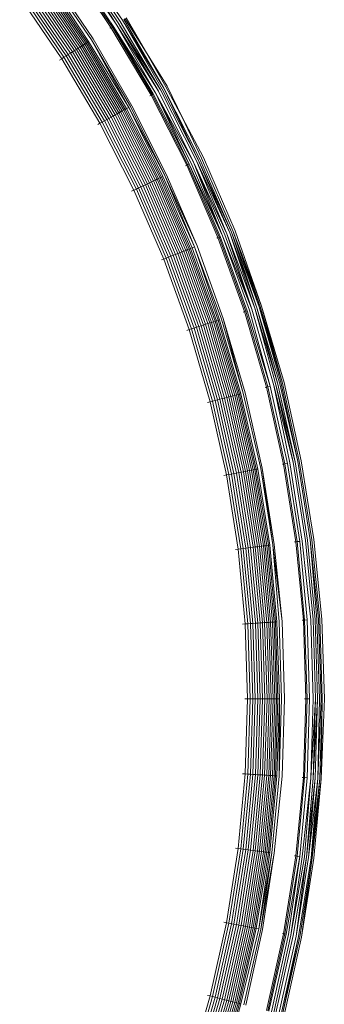
# Model space of a CAD drawing. Units: inches. Extents: x 64 to 1167, y 117 to 939.
# Tile 53 of 56: x 1131.1131 to 1131.3839, y 500.6716 to 501.5456. Entities that reach past the tile are written whole.
import ezdxf

# ---------------------------------------------------------------- set-up
doc = ezdxf.new("R2010")
doc.units = ezdxf.units.IN
doc.header["$MEASUREMENT"] = 0
doc.layers.add('A-FLOR-FIXT', color=8, linetype='Continuous', lineweight=18)

msp = doc.modelspace()

# ---------------------------------------------------------------- linework, layer by layer
at = {"layer": 'A-FLOR-FIXT'}
for p, q in [((1131.20239, 501.54385), (1131.1635, 501.60266)), ((1131.20452, 501.5452), (1131.16482, 501.60362)), ((1131.1943, 501.53871), (1131.15502, 501.5965)), ((1131.19527, 501.53932), (1131.15595, 501.59718)), ((1131.19623, 501.53993), (1131.15687, 501.59785)), ((1131.19902, 501.54171), (1131.15955, 501.59979)), ((1131.19902, 501.54171), (1131.16123, 501.60101)), ((1131.20077, 501.54282), (1131.16123, 501.60101)), ((1131.17837, 501.5286), (1131.13976, 501.58542)), ((1131.1652, 501.52024), (1131.12714, 501.57624)), ((1131.16678, 501.52125), (1131.12865, 501.57735)), ((1131.16829, 501.5222), (1131.1301, 501.57839)), ((1131.16971, 501.52311), (1131.13146, 501.57939)), ((1131.17104, 501.52395), (1131.13274, 501.58031)), ((1131.17228, 501.52474), (1131.13393, 501.58117)), ((1131.17342, 501.52546), (1131.13501, 501.58197)), ((1131.17445, 501.52611), (1131.13688, 501.58332)), ((1131.17686, 501.52764), (1131.13831, 501.58436)), ((1131.15253, 501.5122), (1131.115, 501.56742)), ((1131.15445, 501.51342), (1131.11684, 501.56876)), ((1131.15635, 501.51463), (1131.11866, 501.57009)), ((1131.15822, 501.51581), (1131.12045, 501.57139)), ((1131.16004, 501.51697), (1131.1222, 501.57266)), ((1131.16182, 501.5181), (1131.1239, 501.57389)), ((1131.16354, 501.51919), (1131.12555, 501.57509)), ((1131.15059, 501.51097), (1131.11314, 501.56607)), ((1131.23383, 501.48074), (1131.19902, 501.54171)), ((1131.23659, 501.48226), (1131.19902, 501.54171)), ((1131.23827, 501.48318), (1131.20077, 501.54282)), ((1131.23659, 501.48226), (1131.20077, 501.54282)), ((1131.23827, 501.48318), (1131.20239, 501.54385)), ((1131.23979, 501.48402), (1131.20452, 501.5452)), ((1131.24112, 501.48475), (1131.20452, 501.5452)), ((1131.24112, 501.48475), (1131.20571, 501.54595)), ((1131.22483, 501.51757), (1131.20669, 501.54657)), ((1131.22483, 501.51757), (1131.20771, 501.54722)), ((1131.19332, 501.53809), (1131.1943, 501.53871)), ((1131.1943, 501.53871), (1131.19527, 501.53932)), ((1131.22987, 501.47856), (1131.1943, 501.53871)), ((1131.19527, 501.53932), (1131.19623, 501.53993)), ((1131.23087, 501.47912), (1131.19527, 501.53932)), ((1131.23187, 501.47967), (1131.19623, 501.53993)), ((1131.23383, 501.48074), (1131.19623, 501.53993)), ((1131.16971, 501.52311), (1131.17104, 501.52395)), ((1131.17104, 501.52395), (1131.17228, 501.52474)), ((1131.20573, 501.46529), (1131.17104, 501.52395)), ((1131.17228, 501.52474), (1131.17342, 501.52546)), ((1131.20702, 501.466), (1131.17228, 501.52474)), ((1131.17342, 501.52546), (1131.17445, 501.52611)), ((1131.2082, 501.46665), (1131.17342, 501.52546)), ((1131.21022, 501.46776), (1131.17445, 501.52611)), ((1131.21177, 501.46861), (1131.17686, 501.52764)), ((1131.21022, 501.46776), (1131.17686, 501.52764)), ((1131.21281, 501.46919), (1131.17837, 501.5286)), ((1131.15635, 501.51463), (1131.15822, 501.51581)), ((1131.15822, 501.51581), (1131.16004, 501.51697)), ((1131.19242, 501.45798), (1131.15822, 501.51581)), ((1131.16004, 501.51697), (1131.16182, 501.5181)), ((1131.19432, 501.45902), (1131.16004, 501.51697)), ((1131.16182, 501.5181), (1131.16354, 501.51919)), ((1131.19616, 501.46003), (1131.16182, 501.5181)), ((1131.16354, 501.51919), (1131.1652, 501.52024)), ((1131.19794, 501.46101), (1131.16354, 501.51919)), ((1131.1652, 501.52024), (1131.16678, 501.52125)), ((1131.19966, 501.46196), (1131.1652, 501.52024)), ((1131.16678, 501.52125), (1131.16829, 501.5222)), ((1131.20131, 501.46286), (1131.16678, 501.52125)), ((1131.16829, 501.5222), (1131.16971, 501.52311)), ((1131.20287, 501.46372), (1131.16829, 501.5222)), ((1131.20435, 501.46453), (1131.16971, 501.52311)), ((1131.24314, 501.48586), (1131.22483, 501.51757)), ((1131.24429, 501.48649), (1131.22483, 501.51757)), ((1131.14864, 501.50973), (1131.15059, 501.51097)), ((1131.15059, 501.51097), (1131.15253, 501.5122)), ((1131.1845, 501.45362), (1131.15059, 501.51097)), ((1131.15445, 501.51342), (1131.15253, 501.5122)), ((1131.18652, 501.45473), (1131.15253, 501.5122)), ((1131.15445, 501.51342), (1131.15635, 501.51463)), ((1131.18851, 501.45583), (1131.15445, 501.51342)), ((1131.19049, 501.45691), (1131.15635, 501.51463)), ((1131.26761, 501.41913), (1131.23383, 501.48074)), ((1131.26568, 501.41823), (1131.23383, 501.48074)), ((1131.26366, 501.41728), (1131.23383, 501.48074)), ((1131.26761, 501.41913), (1131.23659, 501.48226)), ((1131.27027, 501.42038), (1131.23827, 501.48318)), ((1131.27184, 501.42112), (1131.23979, 501.48402)), ((1131.27321, 501.42177), (1131.24112, 501.48475)), ((1131.27184, 501.42112), (1131.24112, 501.48475)), ((1131.25772, 501.45841), (1131.24314, 501.48586)), ((1131.25772, 501.45841), (1131.24429, 501.48649)), ((1131.22987, 501.47856), (1131.22886, 501.47801)), ((1131.23087, 501.47912), (1131.22987, 501.47856)), ((1131.26159, 501.4163), (1131.22987, 501.47856)), ((1131.23187, 501.47967), (1131.23087, 501.47912)), ((1131.26263, 501.41679), (1131.23087, 501.47912)), ((1131.26366, 501.41728), (1131.23187, 501.47967)), ((1131.20131, 501.46286), (1131.19966, 501.46196)), ((1131.20287, 501.46372), (1131.20131, 501.46286)), ((1131.2321, 501.40243), (1131.20131, 501.46286)), ((1131.20435, 501.46453), (1131.20287, 501.46372)), ((1131.23372, 501.40319), (1131.20287, 501.46372)), ((1131.20573, 501.46529), (1131.20435, 501.46453)), ((1131.23524, 501.4039), (1131.20435, 501.46453)), ((1131.20702, 501.466), (1131.20573, 501.46529)), ((1131.23667, 501.40458), (1131.20573, 501.46529)), ((1131.2082, 501.46665), (1131.20702, 501.466)), ((1131.238, 501.4052), (1131.20702, 501.466)), ((1131.21022, 501.46776), (1131.2082, 501.46665)), ((1131.23921, 501.40577), (1131.2082, 501.46665)), ((1131.24216, 501.40716), (1131.21022, 501.46776)), ((1131.24032, 501.40629), (1131.21022, 501.46776)), ((1131.24216, 501.40716), (1131.21177, 501.46861)), ((1131.24351, 501.40779), (1131.21281, 501.46919)), ((1131.18652, 501.45473), (1131.1845, 501.45362)), ((1131.18851, 501.45583), (1131.18652, 501.45473)), ((1131.21683, 501.39524), (1131.18652, 501.45473)), ((1131.19049, 501.45691), (1131.18851, 501.45583)), ((1131.21889, 501.39621), (1131.18851, 501.45583)), ((1131.19242, 501.45798), (1131.19049, 501.45691)), ((1131.22093, 501.39717), (1131.19049, 501.45691)), ((1131.19432, 501.45902), (1131.19242, 501.45798)), ((1131.22293, 501.39811), (1131.19242, 501.45798)), ((1131.19616, 501.46003), (1131.19432, 501.45902)), ((1131.22488, 501.39903), (1131.19432, 501.45902)), ((1131.19794, 501.46101), (1131.19616, 501.46003)), ((1131.22679, 501.39992), (1131.19616, 501.46003)), ((1131.19966, 501.46196), (1131.19794, 501.46101)), ((1131.22863, 501.40079), (1131.19794, 501.46101)), ((1131.2304, 501.40163), (1131.19966, 501.46196)), ((1131.27487, 501.42255), (1131.25772, 501.45841)), ((1131.27638, 501.42326), (1131.25772, 501.45841)), ((1131.1845, 501.45362), (1131.18248, 501.45251)), ((1131.21475, 501.39426), (1131.1845, 501.45362)), ((1131.29738, 501.35536), (1131.26761, 501.41913)), ((1131.29354, 501.35384), (1131.26761, 501.41913)), ((1131.29553, 501.35462), (1131.26761, 501.41913)), ((1131.29738, 501.35536), (1131.27027, 501.42038)), ((1131.29987, 501.35634), (1131.27027, 501.42038)), ((1131.29987, 501.35634), (1131.27184, 501.42112)), ((1131.30129, 501.3569), (1131.27184, 501.42112)), ((1131.30129, 501.3569), (1131.27321, 501.42177)), ((1131.30298, 501.35757), (1131.27487, 501.42255)), ((1131.30468, 501.35824), (1131.27638, 501.42326)), ((1131.26159, 501.4163), (1131.26055, 501.41581)), ((1131.26263, 501.41679), (1131.26159, 501.4163)), ((1131.28934, 501.35217), (1131.26159, 501.4163)), ((1131.26366, 501.41728), (1131.26263, 501.41679)), ((1131.29041, 501.3526), (1131.26263, 501.41679)), ((1131.29354, 501.35384), (1131.26366, 501.41728)), ((1131.29147, 501.35302), (1131.26366, 501.41728)), ((1131.29354, 501.35384), (1131.26568, 501.41823)), ((1131.2304, 501.40163), (1131.22863, 501.40079)), ((1131.2321, 501.40243), (1131.2304, 501.40163)), ((1131.25729, 501.33948), (1131.2304, 501.40163)), ((1131.23372, 501.40319), (1131.2321, 501.40243)), ((1131.25904, 501.34018), (1131.2321, 501.40243)), ((1131.23524, 501.4039), (1131.23372, 501.40319)), ((1131.2607, 501.34083), (1131.23372, 501.40319)), ((1131.23667, 501.40458), (1131.23524, 501.4039)), ((1131.26227, 501.34145), (1131.23524, 501.4039)), ((1131.238, 501.4052), (1131.23667, 501.40458)), ((1131.26374, 501.34203), (1131.23667, 501.40458)), ((1131.23921, 501.40577), (1131.238, 501.4052)), ((1131.2651, 501.34257), (1131.238, 501.4052)), ((1131.24032, 501.40629), (1131.23921, 501.40577)), ((1131.26635, 501.34307), (1131.23921, 501.40577)), ((1131.26849, 501.34392), (1131.24032, 501.40629)), ((1131.26849, 501.34392), (1131.24216, 501.40716)), ((1131.27076, 501.34482), (1131.24216, 501.40716)), ((1131.27076, 501.34482), (1131.24351, 501.40779)), ((1131.21475, 501.39426), (1131.21266, 501.39328)), ((1131.21683, 501.39524), (1131.21475, 501.39426)), ((1131.24121, 501.33312), (1131.21475, 501.39426)), ((1131.21889, 501.39621), (1131.21683, 501.39524)), ((1131.24335, 501.33396), (1131.21683, 501.39524)), ((1131.22093, 501.39717), (1131.21889, 501.39621)), ((1131.24547, 501.3348), (1131.21889, 501.39621)), ((1131.22293, 501.39811), (1131.22093, 501.39717)), ((1131.24756, 501.33563), (1131.22093, 501.39717)), ((1131.22488, 501.39903), (1131.22293, 501.39811)), ((1131.24961, 501.33644), (1131.22293, 501.39811)), ((1131.22679, 501.39992), (1131.22488, 501.39903)), ((1131.25162, 501.33724), (1131.22488, 501.39903)), ((1131.22863, 501.40079), (1131.22679, 501.39992)), ((1131.25358, 501.33801), (1131.22679, 501.39992)), ((1131.25547, 501.33876), (1131.22863, 501.40079)), ((1131.32587, 501.2906), (1131.30298, 501.35757)), ((1131.32697, 501.29096), (1131.30298, 501.35757)), ((1131.32812, 501.29134), (1131.30298, 501.35757)), ((1131.32812, 501.29134), (1131.30468, 501.35824)), ((1131.28827, 501.35175), (1131.28934, 501.35217)), ((1131.28934, 501.35217), (1131.29041, 501.3526)), ((1131.31301, 501.28643), (1131.28934, 501.35217)), ((1131.29041, 501.3526), (1131.29147, 501.35302)), ((1131.3141, 501.28678), (1131.29041, 501.3526)), ((1131.31519, 501.28713), (1131.29147, 501.35302)), ((1131.31731, 501.28782), (1131.29354, 501.35384)), ((1131.31934, 501.28848), (1131.29354, 501.35384)), ((1131.31934, 501.28848), (1131.29553, 501.35462)), ((1131.31934, 501.28848), (1131.29738, 501.35536)), ((1131.32213, 501.28939), (1131.29738, 501.35536)), ((1131.32378, 501.28993), (1131.29987, 501.35634)), ((1131.32213, 501.28939), (1131.29987, 501.35634)), ((1131.32587, 501.2906), (1131.30129, 501.3569)), ((1131.32378, 501.28993), (1131.30129, 501.3569)), ((1131.25729, 501.33948), (1131.25904, 501.34018)), ((1131.25904, 501.34018), (1131.2607, 501.34083)), ((1131.28202, 501.27636), (1131.25904, 501.34018)), ((1131.2607, 501.34083), (1131.26227, 501.34145)), ((1131.28371, 501.27691), (1131.2607, 501.34083)), ((1131.26227, 501.34145), (1131.26374, 501.34203)), ((1131.28532, 501.27743), (1131.26227, 501.34145)), ((1131.26374, 501.34203), (1131.2651, 501.34257)), ((1131.28682, 501.27792), (1131.26374, 501.34203)), ((1131.2651, 501.34257), (1131.26635, 501.34307)), ((1131.28821, 501.27837), (1131.2651, 501.34257)), ((1131.26635, 501.34307), (1131.26849, 501.34392)), ((1131.28949, 501.27879), (1131.26635, 501.34307)), ((1131.29065, 501.27916), (1131.26849, 501.34392)), ((1131.29259, 501.27979), (1131.26849, 501.34392)), ((1131.294, 501.28025), (1131.27076, 501.34482)), ((1131.24121, 501.33312), (1131.23906, 501.33227)), ((1131.24335, 501.33396), (1131.24121, 501.33312)), ((1131.26378, 501.27043), (1131.24121, 501.33312)), ((1131.24547, 501.3348), (1131.24335, 501.33396)), ((1131.26596, 501.27114), (1131.24335, 501.33396)), ((1131.24756, 501.33563), (1131.24547, 501.3348)), ((1131.26813, 501.27185), (1131.24547, 501.3348)), ((1131.24961, 501.33644), (1131.24756, 501.33563)), ((1131.27027, 501.27254), (1131.24756, 501.33563)), ((1131.24961, 501.33644), (1131.25162, 501.33724)), ((1131.27237, 501.27322), (1131.24961, 501.33644)), ((1131.25162, 501.33724), (1131.25358, 501.33801)), ((1131.27443, 501.27389), (1131.25162, 501.33724)), ((1131.25358, 501.33801), (1131.25547, 501.33876)), ((1131.27643, 501.27454), (1131.25358, 501.33801)), ((1131.25547, 501.33876), (1131.25729, 501.33948)), ((1131.27837, 501.27517), (1131.25547, 501.33876)), ((1131.28023, 501.27578), (1131.25729, 501.33948)), ((1131.33581, 501.22017), (1131.31731, 501.28782)), ((1131.33895, 501.22098), (1131.31934, 501.28848)), ((1131.34266, 501.22193), (1131.32213, 501.28939)), ((1131.34088, 501.22148), (1131.32213, 501.28939)), ((1131.34266, 501.22193), (1131.32378, 501.28993)), ((1131.34424, 501.22234), (1131.32378, 501.28993)), ((1131.3456, 501.22269), (1131.32587, 501.2906)), ((1131.34672, 501.22297), (1131.32587, 501.2906)), ((1131.34672, 501.22297), (1131.32697, 501.29096)), ((1131.34833, 501.22339), (1131.32812, 501.29134)), ((1131.34672, 501.22297), (1131.32812, 501.29134)), ((1131.29065, 501.27916), (1131.28949, 501.27879)), ((1131.30973, 501.21348), (1131.29065, 501.27916)), ((1131.31171, 501.21399), (1131.29259, 501.27979)), ((1131.31366, 501.21449), (1131.294, 501.28025)), ((1131.31171, 501.21399), (1131.294, 501.28025)), ((1131.31301, 501.28643), (1131.31191, 501.28607)), ((1131.31301, 501.28643), (1131.3141, 501.28678)), ((1131.33251, 501.21933), (1131.31301, 501.28643)), ((1131.3141, 501.28678), (1131.31519, 501.28713)), ((1131.33362, 501.21961), (1131.3141, 501.28678)), ((1131.33581, 501.22017), (1131.31519, 501.28713)), ((1131.26158, 501.26972), (1131.26378, 501.27043)), ((1131.26378, 501.27043), (1131.26596, 501.27114)), ((1131.28237, 501.20645), (1131.26378, 501.27043)), ((1131.26596, 501.27114), (1131.26813, 501.27185)), ((1131.28459, 501.20702), (1131.26596, 501.27114)), ((1131.26813, 501.27185), (1131.27027, 501.27254)), ((1131.2868, 501.20759), (1131.26813, 501.27185)), ((1131.27027, 501.27254), (1131.27237, 501.27322)), ((1131.28898, 501.20815), (1131.27027, 501.27254)), ((1131.27237, 501.27322), (1131.27443, 501.27389)), ((1131.29112, 501.2087), (1131.27237, 501.27322)), ((1131.27643, 501.27454), (1131.27443, 501.27389)), ((1131.29321, 501.20924), (1131.27443, 501.27389)), ((1131.27837, 501.27517), (1131.27643, 501.27454)), ((1131.29525, 501.20976), (1131.27643, 501.27454)), ((1131.28023, 501.27578), (1131.27837, 501.27517)), ((1131.29722, 501.21027), (1131.27837, 501.27517)), ((1131.28202, 501.27636), (1131.28023, 501.27578)), ((1131.29912, 501.21075), (1131.28023, 501.27578)), ((1131.28371, 501.27691), (1131.28202, 501.27636)), ((1131.30094, 501.21122), (1131.28202, 501.27636)), ((1131.28532, 501.27743), (1131.28371, 501.27691)), ((1131.30267, 501.21166), (1131.28371, 501.27691)), ((1131.28682, 501.27792), (1131.28532, 501.27743)), ((1131.3043, 501.21208), (1131.28532, 501.27743)), ((1131.28821, 501.27837), (1131.28682, 501.27792)), ((1131.30583, 501.21248), (1131.28682, 501.27792)), ((1131.28949, 501.27879), (1131.28821, 501.27837)), ((1131.30725, 501.21284), (1131.28821, 501.27837)), ((1131.30855, 501.21318), (1131.28949, 501.27879)), ((1131.33251, 501.21933), (1131.33139, 501.21904)), ((1131.33362, 501.21961), (1131.33251, 501.21933)), ((1131.34775, 501.15113), (1131.33251, 501.21933)), ((1131.33581, 501.22017), (1131.33362, 501.21961)), ((1131.34888, 501.15135), (1131.33362, 501.21961)), ((1131.3511, 501.15177), (1131.33581, 501.22017)), ((1131.35625, 501.15275), (1131.33895, 501.22098)), ((1131.35325, 501.15218), (1131.33895, 501.22098)), ((1131.35625, 501.15275), (1131.34088, 501.22148)), ((1131.35804, 501.1531), (1131.34088, 501.22148)), ((1131.35804, 501.1531), (1131.34266, 501.22193)), ((1131.36037, 501.15354), (1131.34424, 501.22234)), ((1131.36037, 501.15354), (1131.3456, 501.22269)), ((1131.36163, 501.15378), (1131.34672, 501.22297)), ((1131.36336, 501.15411), (1131.34833, 501.22339)), ((1131.29112, 501.2087), (1131.29321, 501.20924)), ((1131.29321, 501.20924), (1131.29525, 501.20976)), ((1131.3079, 501.14353), (1131.29321, 501.20924)), ((1131.29525, 501.20976), (1131.29722, 501.21027)), ((1131.30997, 501.14392), (1131.29525, 501.20976)), ((1131.29722, 501.21027), (1131.29912, 501.21075)), ((1131.31197, 501.14431), (1131.29722, 501.21027)), ((1131.29912, 501.21075), (1131.30094, 501.21122)), ((1131.31389, 501.14467), (1131.29912, 501.21075)), ((1131.30094, 501.21122), (1131.30267, 501.21166)), ((1131.31574, 501.14503), (1131.30094, 501.21122)), ((1131.30267, 501.21166), (1131.3043, 501.21208)), ((1131.31749, 501.14536), (1131.30267, 501.21166)), ((1131.3043, 501.21208), (1131.30583, 501.21248)), ((1131.31915, 501.14568), (1131.3043, 501.21208)), ((1131.30583, 501.21248), (1131.30725, 501.21284)), ((1131.3207, 501.14597), (1131.30583, 501.21248)), ((1131.30725, 501.21284), (1131.30855, 501.21318)), ((1131.32214, 501.14625), (1131.30725, 501.21284)), ((1131.30855, 501.21318), (1131.30973, 501.21348)), ((1131.32346, 501.1465), (1131.30855, 501.21318)), ((1131.32466, 501.14673), (1131.30973, 501.21348)), ((1131.32746, 501.14726), (1131.31171, 501.21399)), ((1131.32863, 501.14749), (1131.31366, 501.21449)), ((1131.28013, 501.20588), (1131.28237, 501.20645)), ((1131.28237, 501.20645), (1131.28459, 501.20702)), ((1131.2969, 501.14143), (1131.28237, 501.20645)), ((1131.28459, 501.20702), (1131.2868, 501.20759)), ((1131.29916, 501.14186), (1131.28459, 501.20702)), ((1131.2868, 501.20759), (1131.28898, 501.20815)), ((1131.3014, 501.14229), (1131.2868, 501.20759)), ((1131.28898, 501.20815), (1131.29112, 501.2087)), ((1131.30361, 501.14271), (1131.28898, 501.20815)), ((1131.30578, 501.14313), (1131.29112, 501.2087)), ((1131.34662, 501.15092), (1131.34775, 501.15113)), ((1131.34775, 501.15113), (1131.34888, 501.15135)), ((1131.35868, 501.08212), (1131.34775, 501.15113)), ((1131.34888, 501.15135), (1131.3511, 501.15177)), ((1131.35982, 501.08226), (1131.34888, 501.15135)), ((1131.36207, 501.08254), (1131.3511, 501.15177)), ((1131.36424, 501.08282), (1131.35325, 501.15218)), ((1131.36726, 501.0832), (1131.35625, 501.15275)), ((1131.36908, 501.08343), (1131.35804, 501.1531)), ((1131.37143, 501.08373), (1131.36037, 501.15354)), ((1131.3727, 501.08389), (1131.36163, 501.15378)), ((1131.37445, 501.08411), (1131.36336, 501.15411)), ((1131.2969, 501.14143), (1131.29463, 501.141)), ((1131.29916, 501.14186), (1131.2969, 501.14143)), ((1131.30732, 501.07563), (1131.2969, 501.14143)), ((1131.3014, 501.14229), (1131.29916, 501.14186)), ((1131.3096, 501.07592), (1131.29916, 501.14186)), ((1131.30361, 501.14271), (1131.3014, 501.14229)), ((1131.31186, 501.0762), (1131.3014, 501.14229)), ((1131.30578, 501.14313), (1131.30361, 501.14271)), ((1131.31409, 501.07648), (1131.30361, 501.14271)), ((1131.3079, 501.14353), (1131.30578, 501.14313)), ((1131.31629, 501.07676), (1131.30578, 501.14313)), ((1131.30997, 501.14392), (1131.3079, 501.14353)), ((1131.31843, 501.07703), (1131.3079, 501.14353)), ((1131.31197, 501.14431), (1131.30997, 501.14392)), ((1131.32052, 501.07729), (1131.30997, 501.14392)), ((1131.31389, 501.14467), (1131.31197, 501.14431)), ((1131.32254, 501.07755), (1131.31197, 501.14431)), ((1131.31574, 501.14503), (1131.31389, 501.14467)), ((1131.32448, 501.0778), (1131.31389, 501.14467)), ((1131.31749, 501.14536), (1131.31574, 501.14503)), ((1131.32635, 501.07803), (1131.31574, 501.14503)), ((1131.31915, 501.14568), (1131.31749, 501.14536)), ((1131.32812, 501.07825), (1131.31749, 501.14536)), ((1131.3207, 501.14597), (1131.31915, 501.14568)), ((1131.32979, 501.07847), (1131.31915, 501.14568)), ((1131.32214, 501.14625), (1131.3207, 501.14597)), ((1131.33136, 501.07866), (1131.3207, 501.14597)), ((1131.32346, 501.1465), (1131.32214, 501.14625)), ((1131.33281, 501.07885), (1131.32214, 501.14625)), ((1131.32466, 501.14673), (1131.32346, 501.1465)), ((1131.33415, 501.07902), (1131.32346, 501.1465)), ((1131.33536, 501.07917), (1131.32466, 501.14673)), ((1131.33819, 501.07953), (1131.32746, 501.14726)), ((1131.33937, 501.07968), (1131.32863, 501.14749)), ((1131.33819, 501.07953), (1131.32863, 501.14749)), ((1131.32448, 501.0778), (1131.32635, 501.07803)), ((1131.32635, 501.07803), (1131.32812, 501.07825)), ((1131.33273, 501.0105), (1131.32635, 501.07803)), ((1131.32812, 501.07825), (1131.32979, 501.07847)), ((1131.33451, 501.01062), (1131.32812, 501.07825)), ((1131.32979, 501.07847), (1131.33136, 501.07866)), ((1131.33619, 501.01072), (1131.32979, 501.07847)), ((1131.33136, 501.07866), (1131.33281, 501.07885)), ((1131.33777, 501.01082), (1131.33136, 501.07866)), ((1131.33281, 501.07885), (1131.33415, 501.07902)), ((1131.33923, 501.01091), (1131.33281, 501.07885)), ((1131.33415, 501.07902), (1131.33536, 501.07917)), ((1131.34058, 501.011), (1131.33415, 501.07902)), ((1131.34179, 501.01107), (1131.33536, 501.07917)), ((1131.34383, 501.0112), (1131.33819, 501.07953)), ((1131.34644, 501.01137), (1131.33819, 501.07953)), ((1131.34644, 501.01137), (1131.33937, 501.07968)), ((1131.35868, 501.08212), (1131.35754, 501.08197)), ((1131.35982, 501.08226), (1131.35868, 501.08212)), ((1131.36526, 501.01255), (1131.35868, 501.08212)), ((1131.36207, 501.08254), (1131.35982, 501.08226)), ((1131.3664, 501.01262), (1131.35982, 501.08226)), ((1131.36866, 501.01276), (1131.36207, 501.08254)), ((1131.37189, 501.01297), (1131.36424, 501.08282)), ((1131.37389, 501.01309), (1131.36726, 501.0832)), ((1131.37572, 501.01321), (1131.36908, 501.08343)), ((1131.37735, 501.01331), (1131.37143, 501.08373)), ((1131.37875, 501.0134), (1131.37143, 501.08373)), ((1131.3799, 501.01347), (1131.3727, 501.08389)), ((1131.38168, 501.01358), (1131.37445, 501.08411)), ((1131.30732, 501.07563), (1131.30503, 501.07534)), ((1131.3096, 501.07592), (1131.30732, 501.07563)), ((1131.31359, 501.0093), (1131.30732, 501.07563)), ((1131.31186, 501.0762), (1131.3096, 501.07592)), ((1131.31589, 501.00944), (1131.3096, 501.07592)), ((1131.31186, 501.0762), (1131.31409, 501.07648)), ((1131.31816, 501.00959), (1131.31186, 501.0762)), ((1131.31409, 501.07648), (1131.31629, 501.07676)), ((1131.3204, 501.00973), (1131.31409, 501.07648)), ((1131.31629, 501.07676), (1131.31843, 501.07703)), ((1131.32261, 501.00987), (1131.31629, 501.07676)), ((1131.31843, 501.07703), (1131.32052, 501.07729)), ((1131.32477, 501.01), (1131.31843, 501.07703)), ((1131.32052, 501.07729), (1131.32254, 501.07755)), ((1131.32687, 501.01013), (1131.32052, 501.07729)), ((1131.32254, 501.07755), (1131.32448, 501.0778)), ((1131.3289, 501.01026), (1131.32254, 501.07755)), ((1131.33086, 501.01039), (1131.32448, 501.0778)), ((1131.31129, 501.00915), (1131.31359, 501.0093)), ((1131.31359, 501.0093), (1131.31589, 501.00944)), ((1131.31568, 500.94271), (1131.31359, 501.0093)), ((1131.31589, 501.00944), (1131.31816, 501.00959)), ((1131.31798, 500.94271), (1131.31589, 501.00944)), ((1131.3204, 501.00973), (1131.31816, 501.00959)), ((1131.32026, 500.94271), (1131.31816, 501.00959)), ((1131.32261, 501.00987), (1131.3204, 501.00973)), ((1131.32251, 500.94271), (1131.3204, 501.00973)), ((1131.32477, 501.01), (1131.32261, 501.00987)), ((1131.32472, 500.94271), (1131.32261, 501.00987)), ((1131.32687, 501.01013), (1131.32477, 501.01)), ((1131.32688, 500.94271), (1131.32477, 501.01)), ((1131.3289, 501.01026), (1131.32687, 501.01013)), ((1131.32899, 500.94271), (1131.32687, 501.01013)), ((1131.33086, 501.01039), (1131.3289, 501.01026)), ((1131.33102, 500.94271), (1131.3289, 501.01026)), ((1131.33273, 501.0105), (1131.33086, 501.01039)), ((1131.33298, 500.94271), (1131.33086, 501.01039)), ((1131.33451, 501.01062), (1131.33273, 501.0105)), ((1131.33486, 500.94271), (1131.33273, 501.0105)), ((1131.33619, 501.01072), (1131.33451, 501.01062)), ((1131.33665, 500.94271), (1131.33451, 501.01062)), ((1131.33777, 501.01082), (1131.33619, 501.01072)), ((1131.33833, 500.94271), (1131.33619, 501.01072)), ((1131.33923, 501.01091), (1131.33777, 501.01082)), ((1131.33991, 500.94271), (1131.33777, 501.01082)), ((1131.34058, 501.011), (1131.33923, 501.01091)), ((1131.34138, 500.94271), (1131.33923, 501.01091)), ((1131.34179, 501.01107), (1131.34058, 501.011)), ((1131.34272, 500.94271), (1131.34058, 501.011)), ((1131.34394, 500.94271), (1131.34179, 501.01107)), ((1131.34598, 500.94271), (1131.34383, 501.0112)), ((1131.34859, 500.94271), (1131.34644, 501.01137)), ((1131.36526, 501.01255), (1131.3641, 501.01248)), ((1131.3664, 501.01262), (1131.36526, 501.01255)), ((1131.36745, 500.94271), (1131.36526, 501.01255)), ((1131.36866, 501.01276), (1131.3664, 501.01262)), ((1131.3686, 500.94271), (1131.3664, 501.01262)), ((1131.37086, 500.94271), (1131.36866, 501.01276)), ((1131.3741, 500.94271), (1131.37189, 501.01297)), ((1131.3761, 500.94271), (1131.37389, 501.01309)), ((1131.37793, 500.94271), (1131.37572, 501.01321)), ((1131.37956, 500.94271), (1131.37735, 501.01331)), ((1131.38097, 500.94271), (1131.37875, 501.0134)), ((1131.38212, 500.94271), (1131.3799, 501.01347)), ((1131.38391, 500.94271), (1131.38168, 501.01358)), ((1131.31568, 500.94271), (1131.31338, 500.94271)), ((1131.31359, 500.87612), (1131.31568, 500.94271)), ((1131.31798, 500.94271), (1131.31568, 500.94271)), ((1131.31589, 500.87597), (1131.31798, 500.94271)), ((1131.32026, 500.94271), (1131.31798, 500.94271)), ((1131.31816, 500.87583), (1131.32026, 500.94271)), ((1131.32251, 500.94271), (1131.32026, 500.94271)), ((1131.3204, 500.87569), (1131.32251, 500.94271)), ((1131.32472, 500.94271), (1131.32251, 500.94271)), ((1131.32261, 500.87555), (1131.32472, 500.94271)), ((1131.32688, 500.94271), (1131.32472, 500.94271)), ((1131.32477, 500.87541), (1131.32688, 500.94271)), ((1131.32687, 500.87528), (1131.32899, 500.94271)), ((1131.32899, 500.94271), (1131.32688, 500.94271)), ((1131.3289, 500.87515), (1131.33102, 500.94271)), ((1131.33102, 500.94271), (1131.32899, 500.94271)), ((1131.33086, 500.87503), (1131.33298, 500.94271)), ((1131.33298, 500.94271), (1131.33102, 500.94271)), ((1131.33273, 500.87491), (1131.33486, 500.94271)), ((1131.33486, 500.94271), (1131.33298, 500.94271)), ((1131.33451, 500.8748), (1131.33665, 500.94271)), ((1131.33665, 500.94271), (1131.33486, 500.94271)), ((1131.33619, 500.87469), (1131.33833, 500.94271)), ((1131.33833, 500.94271), (1131.33665, 500.94271)), ((1131.33777, 500.8746), (1131.33991, 500.94271)), ((1131.33991, 500.94271), (1131.33833, 500.94271)), ((1131.33923, 500.8745), (1131.34138, 500.94271)), ((1131.34138, 500.94271), (1131.33991, 500.94271)), ((1131.34058, 500.87442), (1131.34272, 500.94271)), ((1131.34272, 500.94271), (1131.34138, 500.94271)), ((1131.34179, 500.87434), (1131.34394, 500.94271)), ((1131.34394, 500.94271), (1131.34272, 500.94271)), ((1131.34383, 500.87421), (1131.34598, 500.94271)), ((1131.34383, 500.87421), (1131.34394, 500.94271)), ((1131.34644, 500.87405), (1131.34859, 500.94271)), ((1131.36526, 500.87287), (1131.36745, 500.94271)), ((1131.36745, 500.94271), (1131.3663, 500.94271)), ((1131.3664, 500.87279), (1131.3686, 500.94271)), ((1131.3686, 500.94271), (1131.36745, 500.94271)), ((1131.37086, 500.94271), (1131.3686, 500.94271)), ((1131.36866, 500.87265), (1131.37086, 500.94271)), ((1131.37189, 500.87245), (1131.3741, 500.94271)), ((1131.37189, 500.87245), (1131.3761, 500.94271)), ((1131.37389, 500.87232), (1131.3761, 500.94271)), ((1131.37389, 500.87232), (1131.37793, 500.94271)), ((1131.37572, 500.87221), (1131.37793, 500.94271)), ((1131.37808, 500.87206), (1131.37956, 500.94271)), ((1131.37808, 500.87206), (1131.38097, 500.94271)), ((1131.3799, 500.87194), (1131.38212, 500.94271)), ((1131.38112, 500.87187), (1131.38391, 500.94271)), ((1131.38112, 500.87187), (1131.38212, 500.94271)), ((1131.30732, 500.80979), (1131.31359, 500.87612)), ((1131.3096, 500.8095), (1131.31589, 500.87597)), ((1131.31359, 500.87612), (1131.31129, 500.87626)), ((1131.31186, 500.80921), (1131.31816, 500.87583)), ((1131.31589, 500.87597), (1131.31359, 500.87612)), ((1131.31409, 500.80893), (1131.3204, 500.87569)), ((1131.31816, 500.87583), (1131.31589, 500.87597)), ((1131.31629, 500.80865), (1131.32261, 500.87555)), ((1131.3204, 500.87569), (1131.31816, 500.87583)), ((1131.31843, 500.80838), (1131.32477, 500.87541)), ((1131.32261, 500.87555), (1131.3204, 500.87569)), ((1131.32052, 500.80812), (1131.32687, 500.87528)), ((1131.32254, 500.80787), (1131.3289, 500.87515)), ((1131.32477, 500.87541), (1131.32261, 500.87555)), ((1131.32448, 500.80762), (1131.33086, 500.87503)), ((1131.32687, 500.87528), (1131.32477, 500.87541)), ((1131.32635, 500.80738), (1131.33273, 500.87491)), ((1131.3289, 500.87515), (1131.32687, 500.87528)), ((1131.32812, 500.80716), (1131.33451, 500.8748)), ((1131.33086, 500.87503), (1131.3289, 500.87515)), ((1131.32979, 500.80695), (1131.33619, 500.87469)), ((1131.33273, 500.87491), (1131.33086, 500.87503)), ((1131.33136, 500.80675), (1131.33777, 500.8746)), ((1131.33451, 500.8748), (1131.33273, 500.87491)), ((1131.33281, 500.80657), (1131.33923, 500.8745)), ((1131.33415, 500.8064), (1131.34058, 500.87442)), ((1131.33619, 500.87469), (1131.33451, 500.8748)), ((1131.33536, 500.80625), (1131.34179, 500.87434)), ((1131.33777, 500.8746), (1131.33619, 500.87469)), ((1131.33738, 500.80599), (1131.34383, 500.87421)), ((1131.33923, 500.8745), (1131.33777, 500.8746)), ((1131.34058, 500.87442), (1131.33923, 500.8745)), ((1131.33937, 500.80574), (1131.34644, 500.87405)), ((1131.34179, 500.87434), (1131.34058, 500.87442)), ((1131.35868, 500.8033), (1131.36526, 500.87287)), ((1131.35982, 500.80316), (1131.3664, 500.87279)), ((1131.36207, 500.80287), (1131.36866, 500.87265)), ((1131.3641, 500.87294), (1131.36526, 500.87287)), ((1131.36424, 500.8026), (1131.37189, 500.87245)), ((1131.36526, 500.87287), (1131.3664, 500.87279)), ((1131.36629, 500.80234), (1131.37189, 500.87245)), ((1131.3664, 500.87279), (1131.36866, 500.87265)), ((1131.36819, 500.8021), (1131.37389, 500.87232)), ((1131.36819, 500.8021), (1131.37572, 500.87221)), ((1131.36992, 500.80188), (1131.37572, 500.87221)), ((1131.36992, 500.80188), (1131.37808, 500.87206)), ((1131.37209, 500.80161), (1131.37808, 500.87206)), ((1131.37209, 500.80161), (1131.3799, 500.87194)), ((1131.37324, 500.80146), (1131.3799, 500.87194)), ((1131.37324, 500.80146), (1131.38112, 500.87187)), ((1131.37471, 500.80127), (1131.38112, 500.87187)), ((1131.2969, 500.74398), (1131.30732, 500.80979)), ((1131.29916, 500.74355), (1131.3096, 500.8095)), ((1131.3014, 500.74313), (1131.31186, 500.80921)), ((1131.30361, 500.7427), (1131.31409, 500.80893)), ((1131.30503, 500.81008), (1131.30732, 500.80979)), ((1131.30578, 500.74229), (1131.31629, 500.80865)), ((1131.30732, 500.80979), (1131.3096, 500.8095)), ((1131.3079, 500.74189), (1131.31843, 500.80838)), ((1131.3096, 500.8095), (1131.31186, 500.80921)), ((1131.30997, 500.74149), (1131.32052, 500.80812)), ((1131.31186, 500.80921), (1131.31409, 500.80893)), ((1131.31197, 500.74111), (1131.32254, 500.80787)), ((1131.31389, 500.74074), (1131.32448, 500.80762)), ((1131.31409, 500.80893), (1131.31629, 500.80865)), ((1131.31574, 500.74039), (1131.32635, 500.80738)), ((1131.31629, 500.80865), (1131.31843, 500.80838)), ((1131.31749, 500.74006), (1131.32812, 500.80716)), ((1131.31843, 500.80838), (1131.32052, 500.80812)), ((1131.32052, 500.80812), (1131.32254, 500.80787)), ((1131.32254, 500.80787), (1131.32448, 500.80762)), ((1131.32448, 500.80762), (1131.32635, 500.80738)), ((1131.32635, 500.80738), (1131.32812, 500.80716)), ((1131.32812, 500.80716), (1131.32979, 500.80695)), ((1131.31915, 500.73974), (1131.32979, 500.80695)), ((1131.3207, 500.73944), (1131.33136, 500.80675)), ((1131.32214, 500.73917), (1131.33281, 500.80657)), ((1131.32346, 500.73892), (1131.33415, 500.8064)), ((1131.32572, 500.73848), (1131.33536, 500.80625)), ((1131.32572, 500.73848), (1131.33738, 500.80599)), ((1131.32746, 500.73815), (1131.33738, 500.80599)), ((1131.32746, 500.73815), (1131.33937, 500.80574)), ((1131.329, 500.73786), (1131.33937, 500.80574)), ((1131.32979, 500.80695), (1131.33136, 500.80675)), ((1131.33136, 500.80675), (1131.33281, 500.80657)), ((1131.33281, 500.80657), (1131.33415, 500.8064)), ((1131.33415, 500.8064), (1131.33536, 500.80625)), ((1131.34775, 500.73428), (1131.35868, 500.8033)), ((1131.34888, 500.73407), (1131.35982, 500.80316)), ((1131.35, 500.73385), (1131.36207, 500.80287)), ((1131.35219, 500.73344), (1131.36207, 500.80287)), ((1131.35428, 500.73304), (1131.36424, 500.8026)), ((1131.35428, 500.73304), (1131.36629, 500.80234)), ((1131.35625, 500.73266), (1131.36819, 500.8021)), ((1131.35754, 500.80344), (1131.35868, 500.8033)), ((1131.35868, 500.8033), (1131.35982, 500.80316)), ((1131.35887, 500.73216), (1131.36819, 500.8021)), ((1131.35887, 500.73216), (1131.36992, 500.80188)), ((1131.35982, 500.80316), (1131.36207, 500.80287)), ((1131.36103, 500.73175), (1131.37209, 500.80161)), ((1131.36216, 500.73153), (1131.37324, 500.80146)), ((1131.36362, 500.73126), (1131.37324, 500.80146)), ((1131.36362, 500.73126), (1131.37471, 500.80127)), ((1131.28237, 500.67896), (1131.2969, 500.74398)), ((1131.28459, 500.67839), (1131.29916, 500.74355)), ((1131.2868, 500.67783), (1131.3014, 500.74313)), ((1131.28898, 500.67727), (1131.30361, 500.7427)), ((1131.29112, 500.67672), (1131.30578, 500.74229)), ((1131.29321, 500.67618), (1131.3079, 500.74189)), ((1131.29463, 500.74442), (1131.2969, 500.74398)), ((1131.29525, 500.67566), (1131.30997, 500.74149)), ((1131.2969, 500.74398), (1131.29916, 500.74355)), ((1131.29722, 500.67515), (1131.31197, 500.74111)), ((1131.29912, 500.67466), (1131.31389, 500.74074)), ((1131.29916, 500.74355), (1131.3014, 500.74313)), ((1131.30094, 500.67419), (1131.31574, 500.74039)), ((1131.3014, 500.74313), (1131.30361, 500.7427)), ((1131.30267, 500.67375), (1131.31749, 500.74006)), ((1131.30361, 500.7427), (1131.30578, 500.74229)), ((1131.3043, 500.67333), (1131.31915, 500.73974)), ((1131.30578, 500.74229), (1131.3079, 500.74189)), ((1131.30583, 500.67294), (1131.3207, 500.73944)), ((1131.30725, 500.67257), (1131.32214, 500.73917)), ((1131.3079, 500.74189), (1131.30997, 500.74149)), ((1131.30855, 500.67224), (1131.32346, 500.73892)), ((1131.30973, 500.67194), (1131.32572, 500.73848)), ((1131.30997, 500.74149), (1131.31197, 500.74111)), ((1131.31197, 500.74111), (1131.31389, 500.74074)), ((1131.3125, 500.67123), (1131.32746, 500.73815)), ((1131.31389, 500.74074), (1131.31574, 500.74039)), ((1131.31402, 500.67084), (1131.329, 500.73786)), ((1131.31574, 500.74039), (1131.31749, 500.74006)), ((1131.31749, 500.74006), (1131.31915, 500.73974)), ((1131.31915, 500.73974), (1131.3207, 500.73944)), ((1131.3207, 500.73944), (1131.32214, 500.73917)), ((1131.32214, 500.73917), (1131.32346, 500.73892)), ((1131.32346, 500.73892), (1131.32572, 500.73848)), ((1131.33251, 500.66609), (1131.34775, 500.73428)), ((1131.33362, 500.6658), (1131.34888, 500.73407)), ((1131.33472, 500.66552), (1131.35, 500.73385)), ((1131.33688, 500.66497), (1131.35219, 500.73344)), ((1131.33895, 500.66444), (1131.35428, 500.73304)), ((1131.34088, 500.66394), (1131.35625, 500.73266)), ((1131.34347, 500.66327), (1131.35887, 500.73216)), ((1131.3456, 500.66273), (1131.36103, 500.73175)), ((1131.34775, 500.73428), (1131.34662, 500.7345)), ((1131.34672, 500.66244), (1131.36103, 500.73175)), ((1131.34672, 500.66244), (1131.36216, 500.73153)), ((1131.34888, 500.73407), (1131.34775, 500.73428)), ((1131.34815, 500.66207), (1131.36362, 500.73126)), ((1131.35, 500.73385), (1131.34888, 500.73407)), ((1131.26378, 500.61498), (1131.28237, 500.67896)), ((1131.26596, 500.61427), (1131.28459, 500.67839)), ((1131.26813, 500.61357), (1131.2868, 500.67783)), ((1131.27027, 500.61288), (1131.28898, 500.67727)), ((1131.27237, 500.61219), (1131.29112, 500.67672)), ((1131.27443, 500.61152), (1131.29321, 500.67618)), ((1131.28013, 500.67954), (1131.28237, 500.67896)), ((1131.28237, 500.67896), (1131.28459, 500.67839)), ((1131.28459, 500.67839), (1131.2868, 500.67783)), ((1131.2868, 500.67783), (1131.28898, 500.67727)), ((1131.28898, 500.67727), (1131.29112, 500.67672)), ((1131.29112, 500.67672), (1131.29321, 500.67618)), ((1131.29321, 500.67618), (1131.29525, 500.67566)), ((1131.27643, 500.61087), (1131.29525, 500.67566)), ((1131.27837, 500.61024), (1131.29722, 500.67515)), ((1131.28023, 500.60964), (1131.29912, 500.67466)), ((1131.28202, 500.60906), (1131.30094, 500.67419)), ((1131.28371, 500.60851), (1131.30267, 500.67375)), ((1131.28532, 500.60799), (1131.3043, 500.67333)), ((1131.28682, 500.6075), (1131.30583, 500.67294)), ((1131.28821, 500.60705), (1131.30725, 500.67257)), ((1131.28949, 500.60663), (1131.30855, 500.67224)), ((1131.29169, 500.60592), (1131.30973, 500.67194)), ((1131.29525, 500.67566), (1131.29722, 500.67515)), ((1131.29722, 500.67515), (1131.29912, 500.67466)), ((1131.29912, 500.67466), (1131.30094, 500.67419)), ((1131.30094, 500.67419), (1131.30267, 500.67375)), ((1131.30267, 500.67375), (1131.3043, 500.67333)), ((1131.3043, 500.67333), (1131.30583, 500.67294)), ((1131.30583, 500.67294), (1131.30725, 500.67257)), ((1131.30725, 500.67257), (1131.30855, 500.67224)), ((1131.30855, 500.67224), (1131.30973, 500.67194))]:
    msp.add_line(p, q, dxfattribs=at)

doc.saveas('drawing.dxf')
